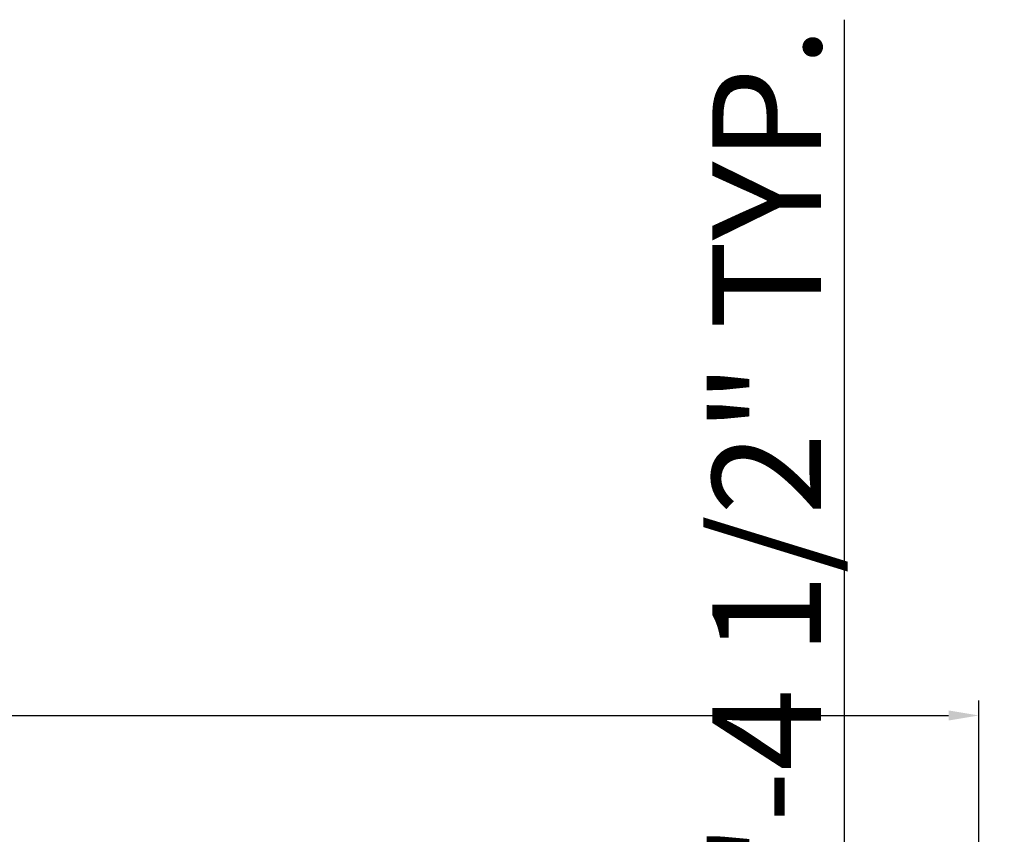
# Model space of a CAD drawing. Units: inches. Extents: x 3590 to 5167, y 65 to 1917.
# Tile 99 of 100: x 5001 to 5082, y 1808 to 1875. Entities that reach past the tile are written whole.
import ezdxf

# ---------------------------------------------------------------- set-up
doc = ezdxf.new("R2010")
doc.units = ezdxf.units.IN
doc.layers.add('A-ANNO-DIMS', color=2, linetype='Continuous', lineweight=18)
doc.styles.get("Standard").update_dxf_attribs({"font": 'arial.ttf'})
doc.dimstyles.new('ISO-25', dxfattribs={"dimtxt": 9, "dimasz": 2.5, "dimexe": 1.25, "dimexo": 0.625, "dimtad": 1, "dimdec": 1, "dimlunit": 3, "dimtxsty": 'Standard', "dimcen": 2.5, "dimadec": 0, "dimazin": 0, "dimtfac": 1, "dimtdec": 1, "dimtmove": 0, "dimatfit": 3, "dimfxl": 1, "dimarcsym": 0})

# ---------------------------------------------------------------- blocks, each defined once
blk = doc.blocks.new('*D101')
at = {"layer": 'A-ANNO-DIMS', "color": 0, "lineweight": -2, "transparency": 16777216}
for p, q in [((4420.274, 1806.624), (4420.274, 1818.615)), ((5080.274, 1806.624), (5080.274, 1818.615)), ((4422.774, 1817.365), (5077.774, 1817.365))]:
    blk.add_line(p, q, dxfattribs=at)
at = {"layer": 'A-ANNO-DIMS', "color": 0, "transparency": 16777216}
for points in [[(4422.774, 1817.781), (4422.774, 1816.948), (4420.274, 1817.365)], [(5077.774, 1817.781), (5077.774, 1816.948), (5080.274, 1817.365)]]:
    blk.add_solid(points, dxfattribs=at)
at = {"layer": 'Defpoints', "color": 0, "transparency": 16777216}
for p in [(5080.274, 1817.365), (4420.274, 1805.999), (5080.274, 1805.999)]:
    blk.add_point(p, dxfattribs=at)
at = {"layer": 'A-ANNO-DIMS', "color": 0, "transparency": 16777216, "insert": (4750.274, 1822.566), "char_height": 9, "attachment_point": 5}
blk.add_mtext("55'", dxfattribs=at)
blk = doc.blocks.new('*D323')
at = {"layer": 'A-ANNO-DIMS', "color": 0, "lineweight": -2, "transparency": 16777216}
for p, q in [((5069.172, 1795.216), (5069.172, 1874.95)), ((5065.437, 1795.216), (5070.422, 1795.216)), ((5069.172, 1769.309), (5069.172, 1792.716)), ((5065.437, 1766.809), (5070.422, 1766.809))]:
    blk.add_line(p, q, dxfattribs=at)
at = {"layer": 'A-ANNO-DIMS', "color": 0, "transparency": 16777216}
for points in [[(5068.756, 1792.716), (5069.589, 1792.716), (5069.172, 1795.216)], [(5068.756, 1769.309), (5069.589, 1769.309), (5069.172, 1766.809)]]:
    blk.add_solid(points, dxfattribs=at)
at = {"layer": 'Defpoints', "color": 0, "transparency": 16777216}
for p in [(5064.812, 1795.216), (5069.172, 1795.216), (5064.812, 1766.809)]:
    blk.add_point(p, dxfattribs=at)
at = {"layer": 'A-ANNO-DIMS', "color": 0, "transparency": 16777216, "insert": (5063.894, 1836.333), "char_height": 9, "attachment_point": 5, "rotation": 90}
blk.add_mtext('2\'-4 1/2" TYP.', dxfattribs=at)

msp = doc.modelspace()

# ---------------------------------------------------------------- dimensions: what is measured, and where the dimension line sits
at = {"layer": 'A-ANNO-DIMS'}
dim = msp.add_linear_dim(base=(5069.172, 1795.216), p1=(5064.812, 1766.809), p2=(5064.812, 1795.216), angle=90, text='<> TYP.', dimstyle='ISO-25', override={"dimdec": 1, "dimlfac": 1, "dimrnd": 0, "dimzin": 1, "dimdsep": 46, "dimlunit": 4, "dimfrac": 2}, dxfattribs=at)
dim.commit()
dim.dimension.update_dxf_attribs({"geometry": '*D323', "text_midpoint": (5063.894, 1836.333)})
dim = msp.add_linear_dim(base=(5080.274, 1817.365), p1=(4420.274, 1805.999), p2=(5080.274, 1805.999), dimstyle='ISO-25', override={"dimclrd": 0, "dimclre": 0, "dimclrt": 0}, dxfattribs=at)
dim.commit()
dim.dimension.update_dxf_attribs({"geometry": '*D101', "text_midpoint": (4750.274, 1822.566)})

doc.saveas('drawing.dxf')
